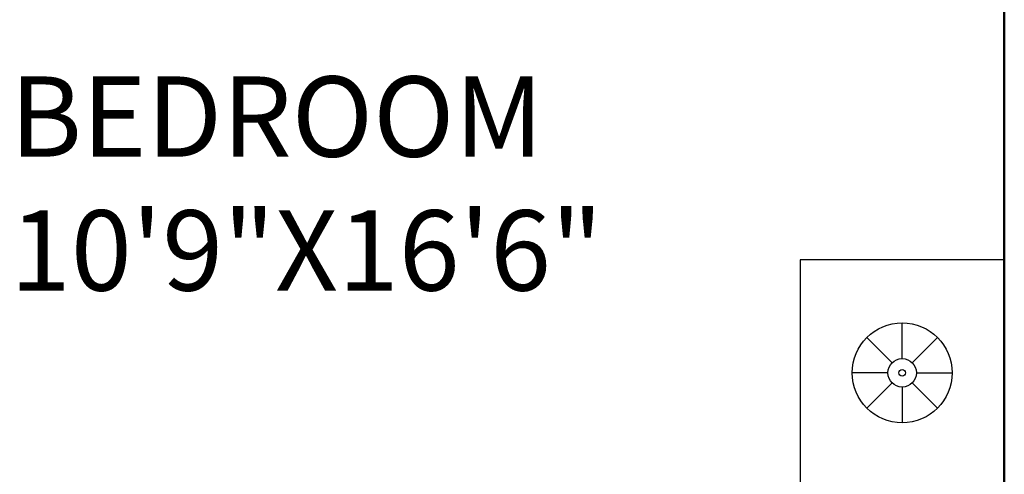
# Model space of a CAD drawing. Units: inches. Extents: x 3064 to 19385, y 846 to 15425.
# Tile 71 of 108: x 6518 to 6604, y 1686 to 1725. Entities that reach past the tile are written whole.
import ezdxf

# ---------------------------------------------------------------- set-up
doc = ezdxf.new("R2010")
doc.units = ezdxf.units.IN
for name, color, linetype, lineweight in [('A-AREA-IDEN', 3, 'Continuous', 18), ('A-FLOR-FIXT', 9, 'Continuous', 18), ('A-WALL', 7, 'Continuous', 50)]:
    doc.layers.add(name, color=color, linetype=linetype, lineweight=lineweight)
doc.layers.add('BLOCK', color=6, linetype='Continuous')
doc.styles.get("Standard").update_dxf_attribs({"font": 'arial.ttf'})

# ---------------------------------------------------------------- blocks, each defined once
blk = doc.blocks.new('A$C52E67D0D')
at = {"layer": 'BLOCK'}
for p, q in [((250.5, 1605.5), (250.5, 1684.7)), ((228.3, 1596.3), (172.3, 1652.3)), ((272.7, 1596.3), (328.7, 1652.3)), ((219.1, 1574.1), (139.9, 1574.1)), ((281.9, 1574.1), (361.1, 1574.1)), ((228.3, 1551.9), (172.3, 1495.9)), ((272.7, 1551.9), (328.7, 1495.9)), ((250.5, 1542.8), (250.5, 1463.5))]:
    blk.add_line(p, q, dxfattribs=at)
blk.add_lwpolyline([(501, 1348.6), (501, 1799.6), (0, 1799.6), (0, 1348.6)], close=True, dxfattribs=at)
for radius in [110.6, 31.4, 7.46]:
    blk.add_circle((250.5, 1574.1), radius, dxfattribs=at)

msp = doc.modelspace()

# ---------------------------------------------------------------- linework, layer by layer
at = {"layer": 'A-WALL'}
msp.add_line((6604.034, 1735.989), (6604.034, 1573.989), dxfattribs=at)

# ---------------------------------------------------------------- block references
at = {"layer": 'A-FLOR-FIXT', "xscale": 0.039370099999992, "yscale": 0.039370099999992, "zscale": 0.039370099999992, "rotation": 270}
msp.add_blockref('A$C52E67D0D', (6533.167, 1704.241), dxfattribs=at)

# ---------------------------------------------------------------- texts
at = {"layer": 'A-AREA-IDEN', "insert": (6517.446, 1720.219), "char_height": 7, "attachment_point": 1}
msp.add_mtext_dynamic_manual_height_columns('BEDROOM\\P10\'9"X16\'6"', width=67.59241, gutter_width=12.5, heights=[0], dxfattribs=at)

doc.saveas('drawing.dxf')
